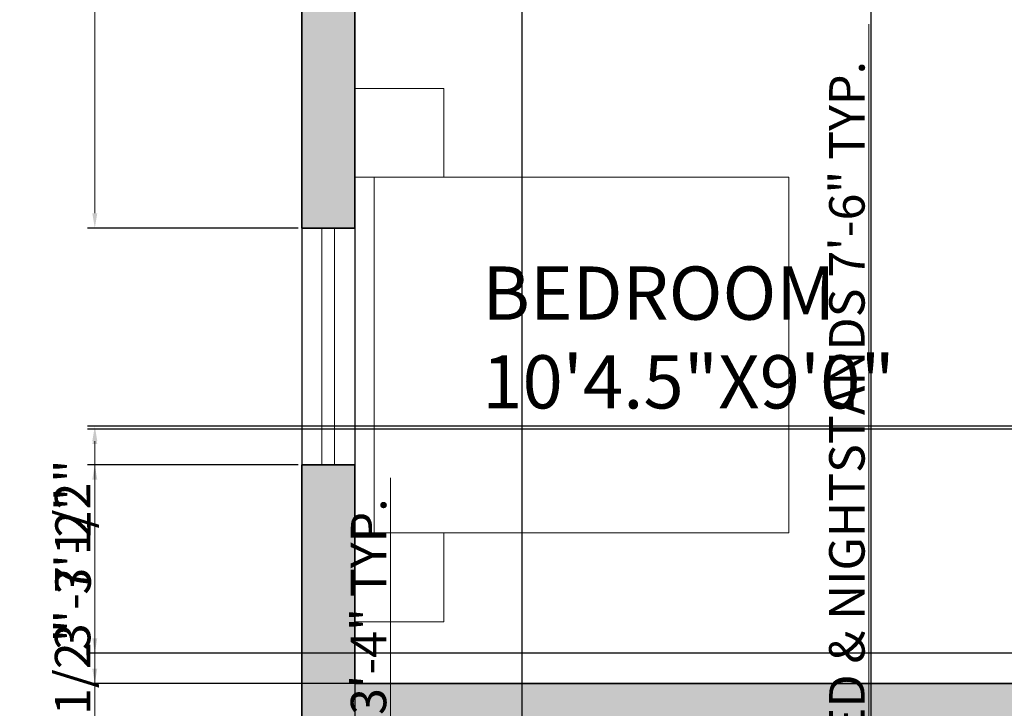
# Model space of a CAD drawing. Units: inches. Extents: x 2696 to 3240, y 1564 to 2310.
# Tile 13 of 76: x 2698 to 2864, y 1736 to 1852. Entities that reach past the tile are written whole.
import ezdxf

# ---------------------------------------------------------------- set-up
doc = ezdxf.new("R2010")
doc.units = ezdxf.units.IN
for name, color, linetype, lineweight in [('A-ANNO-DIMS', 3, 'Continuous', 18), ('A-AREA-IDEN', 7, 'Continuous', 18), ('A-FURN', 251, 'Continuous', 13), ('A-WALL', 7, 'Continuous', 35), ('A-WALL-PATT', 9, 'Continuous', 13), ('WINDOW', 2, 'Continuous', 18)]:
    doc.layers.add(name, color=color, linetype=linetype, lineweight=lineweight)
doc.styles.add('TIMES NEW', font='times.ttf')
doc.styles.add('YQ_DIM', font='SUPEROS.SHX', dxfattribs={"width": 0.8, "bigfont": 'HZDX.SHX'})
doc.dimstyles.new('Siddhuu', dxfattribs={"dimtxt": 6, "dimasz": 2.5, "dimexe": 1.25, "dimexo": 0.625, "dimtad": 1, "dimdec": 1, "dimlunit": 4, "dimtxsty": 'TIMES NEW', "dimcen": 2.5, "dimclrd": 256, "dimclre": 1, "dimclrt": 7, "dimadec": 0, "dimazin": 0, "dimtfac": 1, "dimtdec": 1, "dimtmove": 0, "dimatfit": 3, "dimfxl": 1, "dimtolj": 1, "dimlwd": -1, "dimarcsym": 0})

# ---------------------------------------------------------------- blocks, each defined once
blk = doc.blocks.new('WD_WIN4')
for p, q in [((-0.5, 0.5), (0.5, 0.5)), ((-0.5, 0.12), (0.5, 0.12)), ((-0.5, -0.12), (0.5, -0.12)), ((-0.5, -0.5), (0.5, -0.5))]:
    blk.add_line(p, q)
blk = doc.blocks.new('BED-DOUBLE-WITH-NIGHTSTANDS')
for points in [[(0, 75.13), (0, 90.16), (15.03, 90.16), (15.03, 75.13)], [(3.28, 15.03), (3.28, 75.13), (73.4, 75.13), (73.4, 15.03)], [(0, 15.03), (0, 0), (15.03, 0), (15.03, 15.03)]]:
    blk.add_lwpolyline(points, close=True)
blk = doc.blocks.new('*D22')
at = {"layer": 'A-ANNO-DIMS', "transparency": 16777216}
for p, q in [((2760.61, 1692.7), (2760.61, 1774.98)), ((2760.61, 1655.2), (2760.61, 1690.2))]:
    blk.add_line(p, q, dxfattribs=at)
at = {"layer": 'A-ANNO-DIMS', "color": 1, "lineweight": -2, "transparency": 16777216}
for p, q in [((2755.24, 1692.7), (2761.86, 1692.7)), ((2755.24, 1652.7), (2761.86, 1652.7))]:
    blk.add_line(p, q, dxfattribs=at)
at = {"layer": 'A-ANNO-DIMS', "transparency": 16777216}
for points in [[(2760.19, 1690.2), (2761.03, 1690.2), (2760.61, 1692.7)], [(2760.19, 1655.2), (2761.03, 1655.2), (2760.61, 1652.7)]]:
    blk.add_solid(points, dxfattribs=at)
at = {"layer": 'Defpoints', "color": 0, "transparency": 16777216}
for p in [(2754.61, 1692.7), (2760.61, 1692.7), (2754.61, 1652.7)]:
    blk.add_point(p, dxfattribs=at)
at = {"layer": 'A-ANNO-DIMS', "color": 7, "transparency": 16777216, "insert": (2756.92, 1735.09), "char_height": 6, "attachment_point": 5, "rotation": 90, "style": 'TIMES NEW'}
blk.add_mtext('\\A1;WINDOW 3\'-4" TYP.', dxfattribs=at)
blk = doc.blocks.new('*D46')
at = {"layer": 'A-ANNO-DIMS', "transparency": 16777216}
for p, q in [((2841.54, 1717.22), (2841.54, 1851.66)), ((2841.54, 1629.56), (2841.54, 1714.72))]:
    blk.add_line(p, q, dxfattribs=at)
at = {"layer": 'A-ANNO-DIMS', "color": 1, "lineweight": -2, "transparency": 16777216}
for p, q in [((2828.64, 1717.22), (2842.79, 1717.22)), ((2828.64, 1627.06), (2842.79, 1627.06))]:
    blk.add_line(p, q, dxfattribs=at)
at = {"layer": 'A-ANNO-DIMS', "transparency": 16777216}
for points in [[(2841.12, 1714.72), (2841.96, 1714.72), (2841.54, 1717.22)], [(2841.12, 1629.56), (2841.96, 1629.56), (2841.54, 1627.06)]]:
    blk.add_solid(points, dxfattribs=at)
at = {"layer": 'Defpoints', "color": 0, "transparency": 16777216}
for p in [(2828.01, 1717.22), (2841.54, 1717.22), (2828.01, 1627.06)]:
    blk.add_point(p, dxfattribs=at)
at = {"layer": 'A-ANNO-DIMS', "color": 7, "transparency": 16777216, "insert": (2837.85, 1785.69), "char_height": 6, "attachment_point": 5, "rotation": 90, "style": 'TIMES NEW'}
blk.add_mtext('\\A1;BED & NIGHTSTANDS 7\'-6" TYP.', dxfattribs=at)
blk = doc.blocks.new('*D57')
at = {"layer": 'A-ANNO-DIMS', "color": 1, "lineweight": -2, "transparency": 16777216}
for p, q in [((2754.61, 2018.58), (2754.61, 1568.95)), ((2956.71, 2018.58), (2956.71, 1568.95))]:
    blk.add_line(p, q, dxfattribs=at)
at = {"layer": 'A-ANNO-DIMS', "transparency": 16777216}
blk.add_line((2757.11, 1570.2), (2954.21, 1570.2), dxfattribs=at)
for points in [[(2757.11, 1570.62), (2757.11, 1569.78), (2754.61, 1570.2)], [(2954.21, 1570.62), (2954.21, 1569.78), (2956.71, 1570.2)]]:
    blk.add_solid(points, dxfattribs=at)
at = {"layer": 'Defpoints', "color": 0, "transparency": 16777216}
for p in [(2754.61, 2019.2), (2956.71, 2019.2), (2956.71, 1570.2)]:
    blk.add_point(p, dxfattribs=at)
at = {"layer": 'A-ANNO-DIMS', "color": 7, "transparency": 16777216, "insert": (2855.66, 1573.88), "char_height": 6, "attachment_point": 5, "style": 'TIMES NEW'}
blk.add_mtext('\\A1;16\'-10"', dxfattribs=at)
blk = doc.blocks.new('*D60')
at = {"layer": 'A-ANNO-DIMS', "color": 1, "lineweight": -2, "transparency": 16777216}
for p, q in [((2956.08, 1783.7), (2709.36, 1783.7)), ((2956.08, 1740.2), (2709.36, 1740.2))]:
    blk.add_line(p, q, dxfattribs=at)
at = {"layer": 'A-ANNO-DIMS', "transparency": 16777216}
blk.add_line((2710.61, 1742.7), (2710.61, 1781.2), dxfattribs=at)
for points in [[(2710.19, 1781.2), (2711.03, 1781.2), (2710.61, 1783.7)], [(2710.19, 1742.7), (2711.03, 1742.7), (2710.61, 1740.2)]]:
    blk.add_solid(points, dxfattribs=at)
at = {"layer": 'Defpoints', "color": 0, "transparency": 16777216}
for p in [(2710.61, 1783.7), (2956.71, 1783.7), (2956.71, 1740.2)]:
    blk.add_point(p, dxfattribs=at)
at = {"layer": 'A-ANNO-DIMS', "color": 7, "transparency": 16777216, "insert": (2706.85, 1761.95), "char_height": 6, "attachment_point": 5, "rotation": 90, "style": 'TIMES NEW'}
blk.add_mtext('\\A1;3\'-7 1/2"', dxfattribs=at)
blk = doc.blocks.new('*D68')
at = {"layer": 'A-ANNO-DIMS', "color": 1, "lineweight": -2, "transparency": 16777216}
for p, q in [((2745.61, 2261.58), (2745.61, 1568.95)), ((2782.83, 2261.58), (2782.83, 1568.95))]:
    blk.add_line(p, q, dxfattribs=at)
at = {"layer": 'A-ANNO-DIMS', "transparency": 16777216}
blk.add_line((2748.11, 1570.2), (2780.33, 1570.2), dxfattribs=at)
for points in [[(2748.11, 1570.62), (2748.11, 1569.78), (2745.61, 1570.2)], [(2780.33, 1570.62), (2780.33, 1569.78), (2782.83, 1570.2)]]:
    blk.add_solid(points, dxfattribs=at)
at = {"layer": 'Defpoints', "color": 0, "transparency": 16777216}
for p in [(2745.61, 2262.2), (2782.83, 2262.2), (2782.83, 1570.2)]:
    blk.add_point(p, dxfattribs=at)
at = {"layer": 'A-ANNO-DIMS', "color": 7, "transparency": 16777216, "insert": (2764.22, 1573.88), "char_height": 6, "attachment_point": 5, "style": 'TIMES NEW'}
blk.add_mtext('\\A1;3\'-1"', dxfattribs=at)
blk = doc.blocks.new('*D69')
at = {"layer": 'A-ANNO-DIMS', "color": 1, "lineweight": -2, "transparency": 16777216}
for p, q in [((2841.89, 2261.58), (2841.89, 1568.95)), ((2905.91, 2261.58), (2905.91, 1568.95))]:
    blk.add_line(p, q, dxfattribs=at)
at = {"layer": 'A-ANNO-DIMS', "transparency": 16777216}
blk.add_line((2844.39, 1570.2), (2903.41, 1570.2), dxfattribs=at)
for points in [[(2844.39, 1570.62), (2844.39, 1569.78), (2841.89, 1570.2)], [(2903.41, 1570.62), (2903.41, 1569.78), (2905.91, 1570.2)]]:
    blk.add_solid(points, dxfattribs=at)
at = {"layer": 'Defpoints', "color": 0, "transparency": 16777216}
for p in [(2841.89, 2262.2), (2905.91, 2262.2), (2905.91, 1570.2)]:
    blk.add_point(p, dxfattribs=at)
at = {"layer": 'A-ANNO-DIMS', "color": 7, "transparency": 16777216, "insert": (2873.9, 1573.88), "char_height": 6, "attachment_point": 5, "style": 'TIMES NEW'}
blk.add_mtext('\\A1;5\'-4"', dxfattribs=at)
blk = doc.blocks.new('*D73')
at = {"layer": 'A-ANNO-DIMS', "color": 1, "lineweight": -2, "transparency": 16777216}
for p, q in [((2744.99, 1930.2), (2709.36, 1930.2)), ((2744.99, 1817.2), (2709.36, 1817.2))]:
    blk.add_line(p, q, dxfattribs=at)
at = {"layer": 'A-ANNO-DIMS', "transparency": 16777216}
blk.add_line((2710.61, 1927.7), (2710.61, 1819.7), dxfattribs=at)
for points in [[(2710.19, 1927.7), (2711.03, 1927.7), (2710.61, 1930.2)], [(2710.19, 1819.7), (2711.03, 1819.7), (2710.61, 1817.2)]]:
    blk.add_solid(points, dxfattribs=at)
at = {"layer": 'Defpoints', "color": 0, "transparency": 16777216}
for p in [(2745.61, 1930.2), (2710.61, 1817.2), (2745.61, 1817.2)]:
    blk.add_point(p, dxfattribs=at)
at = {"layer": 'A-ANNO-DIMS', "color": 7, "transparency": 16777216, "insert": (2706.93, 1873.7), "char_height": 6, "attachment_point": 5, "rotation": 90, "style": 'TIMES NEW'}
blk.add_mtext('\\A1;9\'-5"', dxfattribs=at)
blk = doc.blocks.new('*D74')
at = {"layer": 'A-ANNO-DIMS', "color": 1, "lineweight": -2, "transparency": 16777216}
for p, q in [((2744.99, 1777.2), (2709.36, 1777.2)), ((2744.99, 1692.7), (2709.36, 1692.7))]:
    blk.add_line(p, q, dxfattribs=at)
at = {"layer": 'A-ANNO-DIMS', "transparency": 16777216}
blk.add_line((2710.61, 1774.7), (2710.61, 1695.2), dxfattribs=at)
for points in [[(2710.19, 1774.7), (2711.03, 1774.7), (2710.61, 1777.2)], [(2710.19, 1695.2), (2711.03, 1695.2), (2710.61, 1692.7)]]:
    blk.add_solid(points, dxfattribs=at)
at = {"layer": 'Defpoints', "color": 0, "transparency": 16777216}
for p in [(2745.61, 1777.2), (2710.61, 1692.7), (2745.61, 1692.7)]:
    blk.add_point(p, dxfattribs=at)
at = {"layer": 'A-ANNO-DIMS', "color": 7, "transparency": 16777216, "insert": (2706.85, 1734.95), "char_height": 6, "attachment_point": 5, "rotation": 90, "style": 'TIMES NEW'}
blk.add_mtext('\\A1;7\'-0 1/2"', dxfattribs=at)
blk = doc.blocks.new('*D80')
at = {"layer": 'A-ANNO-DIMS', "color": 1, "lineweight": -2, "transparency": 16777216}
for p, q in [((3198.99, 1783.2), (2709.36, 1783.2)), ((3198.99, 1745.35), (2709.36, 1745.35))]:
    blk.add_line(p, q, dxfattribs=at)
at = {"layer": 'A-ANNO-DIMS', "transparency": 16777216}
blk.add_line((2710.61, 1780.7), (2710.61, 1747.85), dxfattribs=at)
for points in [[(2710.19, 1780.7), (2711.03, 1780.7), (2710.61, 1783.2)], [(2710.19, 1747.85), (2711.03, 1747.85), (2710.61, 1745.35)]]:
    blk.add_solid(points, dxfattribs=at)
at = {"layer": 'Defpoints', "color": 0, "transparency": 16777216}
for p in [(3199.61, 1783.2), (2710.61, 1745.35), (3199.61, 1745.35)]:
    blk.add_point(p, dxfattribs=at)
at = {"layer": 'A-ANNO-DIMS', "color": 7, "transparency": 16777216, "insert": (2706.93, 1764.28), "char_height": 6, "attachment_point": 5, "rotation": 90, "style": 'TIMES NEW'}
blk.add_mtext('\\A1;3\'-2"', dxfattribs=at)

msp = doc.modelspace()

# ---------------------------------------------------------------- hatches: boundary and pattern name
at = {"layer": 'A-WALL-PATT', "transparency": 33554556}
h = msp.add_hatch(color=256, dxfattribs=at)
h.dxf.hatch_style = 1
h.paths.add_polyline_path([(2879.11, 2253.2), (2905.91, 2253.2), (2905.91, 2262.2), (2841.89, 2262.2), (2841.89, 2253.2), (2870.11, 2253.2), (2870.11, 2176.6), (2965.71, 2176.6), (2965.71, 2206.7), (2973.58, 2206.7), (2973.58, 2215.7), (2965.71, 2215.7), (2965.71, 2262.2), (2929.91, 2262.2), (2929.91, 2253.2), (2956.71, 2253.2), (2956.71, 2185.6), (2879.11, 2185.6)])
h.paths.add_polyline_path([(2782.83, 2262.2), (2745.61, 2262.2), (2745.61, 2228.73), (2754.61, 2228.73), (2754.61, 2253.2), (2782.83, 2253.2)])
h.paths.add_polyline_path([(2754.61, 2136.2), (2965.71, 2136.2), (2965.71, 2145.2), (2879.11, 2145.2), (2879.11, 2147.07), (2877.34, 2147.07), (2870.11, 2147.07), (2870.11, 2145.2), (2754.61, 2145.2), (2754.61, 2169.67), (2745.61, 2169.67), (2745.61, 2000.2), (2754.61, 2000.2), (2754.61, 2019.2), (2849.08, 2019.2), (2849.08, 2023.7), (2841.21, 2023.7), (2841.21, 2051.83), (2836.71, 2051.83), (2836.71, 2023.7), (2754.61, 2023.7), (2754.61, 2091.2), (2836.71, 2091.2), (2836.71, 2087.83), (2841.21, 2087.83), (2841.21, 2095.7), (2754.61, 2095.7)])
h.paths.add_polyline_path([(2965.71, 2136.2), (2956.71, 2136.2), (2956.71, 2023.7), (2885.08, 2023.7), (2885.08, 2019.2), (2956.71, 2019.2), (2956.71, 1950.58), (2965.71, 1950.58), (2965.71, 1980.2), (2973.58, 1980.2), (2973.58, 1989.2), (2965.71, 1989.2)])
h.paths.add_polyline_path([(2754.61, 1906.7), (2880.21, 1906.7), (2884.71, 1906.7), (2956.71, 1906.7), (2956.71, 1792.7), (2944.71, 1792.7), (2944.71, 1783.7), (2956.71, 1783.7), (2956.71, 1740.2), (2884.71, 1740.2), (2884.71, 1783.7), (2896.71, 1783.7), (2896.71, 1792.7), (2884.71, 1792.7), (2884.71, 1846.7), (2880.21, 1846.7), (2880.21, 1740.2), (2754.61, 1740.2), (2754.61, 1777.2), (2745.61, 1777.2), (2745.61, 1692.7), (2754.61, 1692.7), (2754.61, 1731.2), (2956.71, 1731.2), (2956.71, 1723.33), (2965.71, 1723.33), (2965.71, 1884.2), (2973.58, 1884.2), (2973.58, 1893.2), (2965.71, 1893.2), (2965.71, 1914.58), (2956.71, 1914.58), (2956.71, 1911.2), (2754.61, 1911.2), (2754.61, 1930.2), (2745.61, 1930.2), (2745.61, 1817.2), (2754.61, 1817.2), (2754.61, 1854.2), (2826.61, 1854.2), (2826.61, 1868.83), (2822.11, 1868.83), (2822.11, 1858.7), (2754.61, 1858.7)])
h.paths.add_polyline_path([(2965.71, 1656.2), (3008.24, 1656.2), (3008.24, 1665.2), (2965.71, 1665.2), (2965.71, 1693.33), (2956.71, 1693.33), (2956.71, 1686.2), (2934.58, 1686.2), (2934.58, 1681.7), (2956.71, 1681.7), (2956.71, 1614.2), (2896.71, 1614.2), (2896.71, 1681.7), (2904.58, 1681.7), (2904.58, 1686.2), (2892.21, 1686.2), (2892.21, 1614.2), (2858.41, 1614.2), (2858.41, 1605.2), (2965.71, 1605.2)])
h.paths.add_polyline_path([(2788.41, 1614.2), (2754.61, 1614.2), (2754.61, 1652.7), (2745.61, 1652.7), (2745.61, 1605.2), (2788.41, 1605.2)])
h.paths.add_polyline_path([(3199.61, 1633.05), (3190.61, 1633.05), (3190.61, 1614.2), (3082.61, 1614.2), (3082.61, 1665.2), (3070.24, 1665.2), (3070.24, 1656.2), (3078.11, 1656.2), (3078.11, 1605.2), (3199.61, 1605.2)])
h.paths.add_polyline_path([(3199.61, 1702.05), (3190.61, 1702.05), (3190.61, 1699.7), (3106.61, 1699.7), (3106.61, 1747.7), (3190.61, 1747.7), (3190.61, 1752.2), (3082.61, 1752.2), (3082.61, 1760.08), (3078.11, 1760.08), (3078.11, 1747.7), (3102.11, 1747.7), (3102.11, 1699.7), (3078.11, 1699.7), (3078.11, 1695.2), (3190.61, 1695.2), (3190.61, 1676.35), (3199.61, 1676.35)])
h.paths.add_polyline_path([(3199.61, 1783.2), (3190.61, 1783.2), (3190.61, 1745.35), (3199.61, 1745.35)])
h.paths.add_polyline_path([(3082.61, 1884.2), (3190.61, 1884.2), (3190.61, 1853.2), (3199.61, 1853.2), (3199.61, 1901.7), (3190.61, 1901.7), (3190.61, 1893.2), (3005.58, 1893.2), (3005.58, 1891.28), (3005.58, 1884.2), (3078.11, 1884.2), (3078.11, 1792.08), (3082.61, 1792.08)])
h.paths.add_polyline_path([(3199.61, 1994.7), (3190.61, 1994.7), (3190.61, 1989.2), (3073.71, 1989.2), (3073.71, 2034.2), (3069.21, 2034.2), (3069.21, 1989.2), (3005.58, 1989.2), (3005.58, 1980.2), (3190.61, 1980.2), (3190.61, 1971.7), (3199.61, 1971.7)])
h.paths.add_polyline_path([(3199.61, 2155.2), (3190.61, 2155.2), (3190.61, 2064.7), (3199.61, 2064.7)])
h.paths.add_polyline_path([(3190.61, 2074.7), (3106.61, 2074.7), (3106.61, 2122.7), (3190.61, 2122.7), (3190.61, 2127.2), (3082.71, 2127.2), (3082.71, 2135.08), (3073.71, 2135.08), (3073.71, 2122.7), (3102.11, 2122.7), (3102.11, 2074.7), (3069.21, 2074.7), (3069.21, 2070.2), (3190.61, 2070.2)])
h.paths.add_polyline_path([(3082.71, 2253.2), (3190.61, 2253.2), (3190.61, 2225.2), (3199.61, 2225.2), (3199.61, 2262.2), (3073.71, 2262.2), (3073.71, 2215.7), (3035.58, 2215.7), (3035.58, 2206.7), (3073.71, 2206.7), (3073.71, 2171.08), (3082.71, 2171.08)])

# ---------------------------------------------------------------- linework, layer by layer
at = {"layer": 'A-WALL'}
for p, q in [((2745.61, 1817.2), (2745.61, 1930.2)), ((2754.61, 1817.2), (2754.61, 1854.2)), ((2754.61, 1817.2), (2745.61, 1817.2)), ((2754.61, 1777.2), (2745.61, 1777.2)), ((2745.61, 1692.7), (2745.61, 1777.2)), ((2754.61, 1740.2), (2754.61, 1777.2)), ((2754.61, 1740.2), (2880.21, 1740.2))]:
    msp.add_line(p, q, dxfattribs=at)

# ---------------------------------------------------------------- block references
at = {"layer": 'A-FURN'}
msp.add_blockref('BED-DOUBLE-WITH-NIGHTSTANDS', (2754.61, 1750.66), dxfattribs=at)
at = {"layer": 'WINDOW', "xscale": 40, "yscale": 9, "zscale": 40, "rotation": 270}
msp.add_blockref('WD_WIN4', (2750.11, 1797.2), dxfattribs=at)

# ---------------------------------------------------------------- texts
at = {"layer": 'A-AREA-IDEN', "insert": (2776.16, 1810.71), "char_height": 9, "attachment_point": 1, "style": 'YQ_DIM'}
msp.add_mtext_dynamic_manual_height_columns('BEDROOM\\P10\'4.5"X9\'0"', width=48.0032, gutter_width=12.5, heights=[0], dxfattribs=at)

# ---------------------------------------------------------------- dimensions: what is measured, and where the dimension line sits
at = {"layer": 'A-ANNO-DIMS'}
for base, p1, p2, picture, middle in [((2782.83, 1570.2), (2745.61, 2262.2), (2782.83, 2262.2), '*D68', (2764.22, 1573.88)), ((2905.91, 1570.2), (2841.89, 2262.2), (2905.91, 2262.2), '*D69', (2873.9, 1573.88)), ((2956.71, 1570.2), (2754.61, 2019.2), (2956.71, 2019.2), '*D57', (2855.66, 1573.88))]:
    dim = msp.add_linear_dim(base=base, p1=p1, p2=p2, dimstyle='Siddhuu', override={"dimdec": 1, "dimlfac": 1, "dimrnd": 0, "dimzin": 1, "dimdsep": 46, "dimlunit": 4, "dimfrac": 2}, dxfattribs=at)
    dim.commit()
    dim.dimension.update_dxf_attribs({"geometry": picture, "text_midpoint": middle})
for base, p1, p2, picture, middle in [((2710.61, 1817.2), (2745.61, 1930.2), (2745.61, 1817.2), '*D73', (2706.93, 1873.7)), ((2710.61, 1783.7), (2956.71, 1740.2), (2956.71, 1783.7), '*D60', (2706.85, 1761.95)), ((2710.6114, 1745.3546), (3199.6114, 1783.2011), (3199.6114, 1745.3546), '*D80', (2706.9345, 1764.2779)), ((2710.61, 1692.7), (2745.61, 1777.2), (2745.61, 1692.7), '*D74', (2706.85, 1734.95))]:
    dim = msp.add_linear_dim(base=base, p1=p1, p2=p2, angle=90, dimstyle='Siddhuu', override={"dimdec": 1, "dimlfac": 1, "dimrnd": 0, "dimzin": 1, "dimdsep": 46, "dimlunit": 4, "dimfrac": 2}, dxfattribs=at)
    dim.commit()
    dim.dimension.update_dxf_attribs({"geometry": picture, "text_midpoint": middle})
for base, p1, p2, text, picture, middle in [((2841.54, 1717.22), (2828.01, 1627.06), (2828.01, 1717.22), 'BED & NIGHTSTANDS <> TYP.', '*D46', (2837.85, 1785.69)), ((2760.61, 1692.7), (2754.61, 1652.7), (2754.61, 1692.7), 'WINDOW <> TYP.', '*D22', (2756.92, 1735.09))]:
    dim = msp.add_linear_dim(base=base, p1=p1, p2=p2, angle=90, text=text, dimstyle='Siddhuu', override={"dimdec": 1, "dimlfac": 1, "dimrnd": 0, "dimzin": 1, "dimdsep": 46, "dimlunit": 4, "dimfrac": 2}, dxfattribs=at)
    dim.commit()
    dim.dimension.update_dxf_attribs({"geometry": picture, "text_midpoint": middle})

doc.saveas('drawing.dxf')
